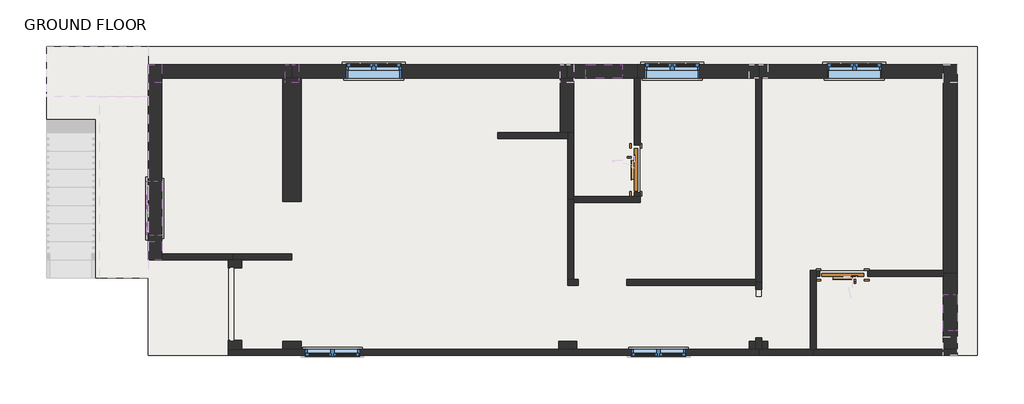
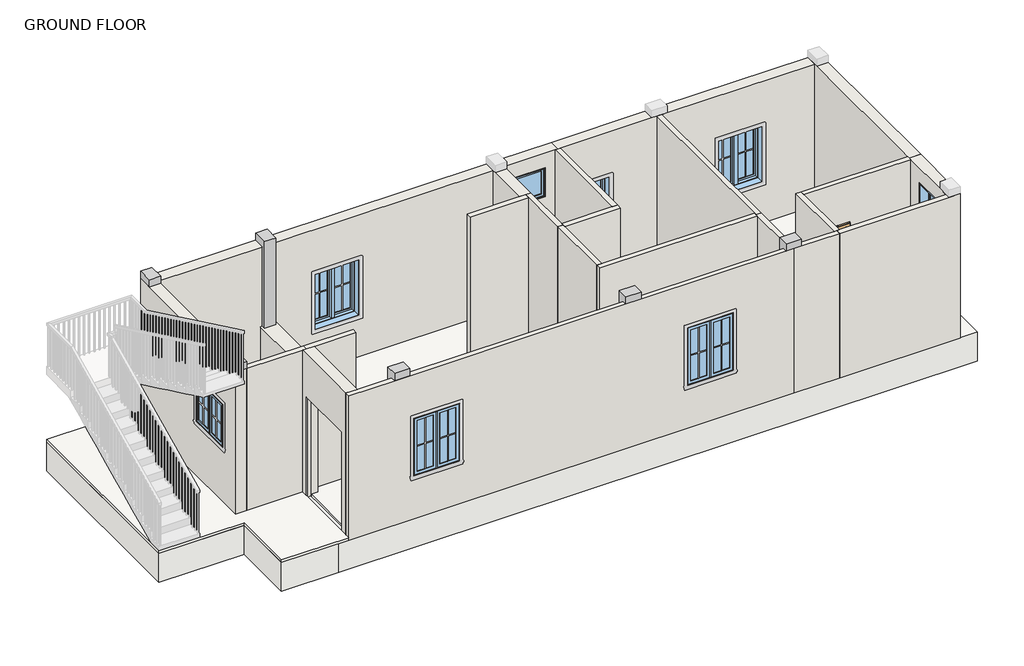
# One storey, part 1 of 3: 26 walls, 8 windows, 6 columns, 4 slabs, 2 doors.
"""IFC4 building model written with IfcOpenShell, lengths in millimetres."""

from ifc_helpers import new_model, si_unit, frame, origin, origin_with_axes, place, context, project, spatial, polyline, outline, extrude, faceted_brep, transform, mapped, element, save
from components import apartment_toilet_door_15897_d3_toilet_d7560075, apartment_toilet_door_15897_d3_toilet_03746f18, window_80340324, window_casement_double_w1_d341e8ac, window_casement_double_w1_80f1179f, window_casement_double_w1_2_90de19e9

model = new_model("IFC4")

# Units and contexts
model_context = context("Model", 3, world=origin())
ifc_project = project(units=[si_unit("LENGTHUNIT", "METRE", prefix="MILLI")], contexts=[model_context])

# Site, building, storey
site = spatial("IfcSite", under=ifc_project)
building = spatial("IfcBuilding", under=site)
storey = spatial("IfcBuildingStorey", under=building, Name="GROUND FLOOR", Elevation=0.0)

# Columns
placement = place(None, origin())
element("IfcColumn", 1, ObjectType="Rectangular Column : 9\" X 12\"", at=placement, inside=storey, context=model_context, shape_type="Brep", body=[
    faceted_brep([(-2166.0591227, 4797.7642852, 3200.4), (-2394.6591227, 4797.7642852, 3200.4), (-2394.6591227, 4797.7642852, 1371.6), (-2166.0591227, 4797.7642852, 1371.6), (-2394.6591227, 5102.5642852, 3200.4), (-2394.6591227, 5102.5642852, 3048.0), (-2394.6591227, 4873.9642852, 3048.0), (-2394.6591227, 4873.9642852, 1371.6), (-2166.0591227, 5102.5642852, 3200.4), (-2166.0591227, 5102.5642852, 3048.0), (-2280.3591227, 5102.5642852, 3048.0), (-2166.0591227, 4873.9642852, 1371.6), (-2166.0591227, 4873.9642852, 3048.0), (-2280.3591227, 4873.9642852, 3048.0), (-2280.3591227, 4873.9642852, 1371.6)], [[[0, 1, 2, 3]], [[1, 4, 5, 6, 7, 2]], [[4, 8, 9, 10, 5]], [[8, 0, 3, 11, 12, 9]], [[1, 0, 8, 4]], [[6, 13, 14, 7]], [[13, 6, 5, 10]], [[13, 12, 11, 14]], [[12, 13, 10, 9]], [[3, 2, 7, 14, 11]]]),
])
element("IfcColumn", 2, ObjectType="Rectangular Column : 9\" X 12\"", at=placement, inside=storey, context=model_context, shape_type="SweptSolid", body=[
    extrude(outline(polyline([(-4693.3591227, 5102.5642852), (-4464.7591227, 5102.5642852), (-4464.7591227, 4797.7642852), (-4693.3591227, 4797.7642852), (-4693.3591227, 5102.5642852)])), frame((0.0, 0.0, 3048.0), z_axis=(0.0, 0.0, 1.0), x_axis=(1.0, 0.0, 0.0)), (0.0, 0.0, 1.0), 152.4),
])
element("IfcColumn", 3, ObjectType="Rectangular Column : 9\" X 12\"", at=placement, inside=storey, context=model_context, shape_type="Brep", body=[
    faceted_brep([(5492.0408773, 454.3642852, 0.0), (5492.0408773, 327.3642852, 0.0), (5390.4408773, 327.3642852, 0.0), (5390.4408773, 454.3642852, 0.0), (5695.2408773, 454.3642852, 3200.4), (5695.2408773, 225.7642852, 3200.4), (5695.2408773, 225.7642852, 3048.0), (5695.2408773, 327.3642852, 3048.0), (5695.2408773, 327.3642852, 0.0), (5695.2408773, 454.3642852, 0.0), (5390.4408773, 225.7642852, 3200.4), (5390.4408773, 225.7642852, 3048.0), (5542.8408773, 225.7642852, 3048.0), (5390.4408773, 454.3642852, 3200.4), (5390.4408773, 327.3642852, 3048.0), (5593.6408773, 454.3642852, 0.0), (5593.6408773, 454.3642852, 3048.0), (5492.0408773, 454.3642852, 3048.0), (5593.6408773, 327.3642852, 3048.0), (5593.6408773, 327.3642852, 0.0), (5492.0408773, 327.3642852, 3048.0), (5542.8408773, 327.3642852, 3048.0)], [[[0, 1, 2, 3]], [[4, 5, 6, 7, 8, 9]], [[5, 10, 11, 12, 6]], [[10, 13, 3, 2, 14, 11]], [[4, 9, 15, 16, 17, 0, 3, 13]], [[5, 4, 13, 10]], [[18, 16, 15, 19]], [[17, 20, 1, 0]], [[16, 18, 21, 20, 17]], [[20, 14, 2, 1]], [[14, 20, 21, 12, 11]], [[7, 18, 19, 8]], [[18, 7, 6, 12, 21]], [[19, 15, 9, 8]]]),
])
element("IfcColumn", 4, ObjectType="Rectangular Column : 9\" X 12\"", at=placement, inside=storey, context=model_context, shape_type="SweptSolid", body=[
    extrude(outline(polyline([(225.7642852, 3200.4), (454.3642852, 3200.4), (454.3642852, 0.0), (327.3642852, 0.0), (327.3642852, 3048.0), (225.7642852, 3048.0), (225.7642852, 3200.4)])), frame((2190.0408773, 0.0, 0.0), z_axis=(1.0, 0.0, 0.0), x_axis=(0.0, 1.0, 0.0)), (0.0, 0.0, 1.0), 304.8),
])
element("IfcColumn", 5, ObjectType="Rectangular Column : 9\" X 12\"", at=placement, inside=storey, context=model_context, shape_type="SweptSolid", body=[
    extrude(outline(polyline([(225.7642852, 3200.4), (454.3642852, 3200.4), (454.3642852, 0.0), (327.3642852, 0.0), (327.3642852, 3048.0), (225.7642852, 3048.0), (225.7642852, 3200.4)])), frame((-2432.7591227, 0.0, 0.0), z_axis=(1.0, 0.0, 0.0), x_axis=(0.0, 1.0, 0.0)), (0.0, 0.0, 1.0), 304.8),
])
element("IfcColumn", 6, ObjectType="Rectangular Column : 9\" X 12\"", at=placement, inside=storey, context=model_context, shape_type="SweptSolid", body=[
    extrude(outline(polyline([(-4693.3591227, 2130.7642852), (-4464.7591227, 2130.7642852), (-4464.7591227, 1825.9642852), (-4693.3591227, 1825.9642852), (-4693.3591227, 2130.7642852)])), frame((0.0, 0.0, 3048.0), z_axis=(0.0, 0.0, 1.0), x_axis=(1.0, 0.0, 0.0)), (0.0, 0.0, 1.0), 152.4),
])

# Doors
apartment_toilet_door_15897_d3_toilet_shape = apartment_toilet_door_15897_d3_toilet_d7560075(model_context)
element("IfcDoor", 7, ObjectType="Apartment_Toilet_Door_15897 : D3 TOILET", at=placement, inside=storey, context=model_context, shape_type="MappedRepresentation", body=[
    mapped(apartment_toilet_door_15897_d3_toilet_shape, transform((6952.5408773, 1597.3642852, 0.0), x_axis=(-1.0, 0.0, 0.0), y_axis=(0.0, -1.0, 0.0), z_axis=(0.0, 0.0, 1.0))),
])
apartment_toilet_door_15897_d3_toilet_2_shape = apartment_toilet_door_15897_d3_toilet_03746f18(model_context)
element("IfcDoor", 8, ObjectType="Apartment_Toilet_Door_15897 : D3 TOILET", at=placement, inside=storey, context=model_context, shape_type="MappedRepresentation", body=[
    mapped(apartment_toilet_door_15897_d3_toilet_2_shape, transform((3510.8408773, 3337.2642852, 0.0), x_axis=(0.0, -1.0, 0.0), y_axis=(1.0, 0.0, 0.0), z_axis=(0.0, 0.0, 1.0))),
])

# Slabs
element("IfcSlab", 9, ObjectType="FLOORING", at=placement, inside=storey, context=model_context, shape_type="SweptSolid", body=[
    extrude(outline(polyline([(-4464.7591227, 1927.5642852), (-4464.7591227, 4873.9642852), (-2432.7591227, 4873.9642852), (-2432.7591227, 2803.8642852), (-2127.9591227, 2803.8642852), (-2127.9591227, 4873.9642852), (2215.4408773, 4873.9642852), (2215.4408773, 3959.5642852), (1174.0408773, 3959.5642852), (1174.0408773, 3857.9642852), (2342.4408773, 3857.9642852), (2342.4408773, 1394.1642852), (2520.2408773, 1394.1642852), (2520.2408773, 1495.7642852), (2444.0408773, 1495.7642852), (2444.0408773, 2791.1642852), (3561.6408773, 2791.1642852), (3561.6408773, 4873.9642852), (5492.0408773, 4873.9642852), (5492.0408773, 1495.7642852), (3409.2408773, 1495.7642852), (3333.0408773, 1495.7642852), (3333.0408773, 1394.1642852), (5492.0408773, 1394.1642852), (5492.0408773, 1203.6642852), (5593.6408773, 1203.6642852), (5593.6408773, 4873.9642852), (8641.6408773, 4873.9642852), (8641.6408773, 1648.1642852), (6406.4408773, 1648.1642852), (6406.4408773, 327.3642852), (5593.6408773, 327.3642852), (5593.6408773, 390.8642852), (5492.0408773, 390.8642852), (5492.0408773, 327.3642852), (-3118.5591227, 327.3642852), (-3118.5591227, 397.6642852), (-3250.1591227, 397.6642852), (-3250.1591227, 1769.2642852), (-3118.5591227, 1769.2642852), (-3118.5591227, 1825.9642852), (-2280.3591227, 1825.9642852), (-2280.3591227, 1927.5642852), (-4464.7591227, 1927.5642852)])), origin_with_axes(), (0.0, 0.0, 1.0), 50.8),
])
element("IfcSlab", 10, ObjectType="FLOORING OPEN AREA", at=placement, inside=storey, context=model_context, shape_type="SweptSolid", body=[
    extrude(outline(polyline([(-4693.3591227, 225.7642852), (-4693.3591227, 1521.1642852), (-6395.1591227, 1521.1642852), (-6395.1591227, 5407.3642852), (-4693.3591227, 5407.3642852), (-4693.3591227, 1825.9642852), (-3347.1591227, 1825.9642852), (-3347.1591227, 225.7642852), (-4693.3591227, 225.7642852)])), origin_with_axes(), (0.0, 0.0, 1.0), 50.8),
])
element("IfcSlab", 11, ObjectType="FLOORING TOILET", at=placement, inside=storey, context=model_context, shape_type="SweptSolid", body=[
    extrude(outline(polyline([(7371.5408773, 1546.5642852), (8641.6408773, 1546.5642852), (8641.6408773, 327.3642852), (6508.0408773, 327.3642852), (6508.0408773, 1546.5642852), (6571.5408773, 1546.5642852), (6571.5408773, 1648.1642852), (7371.5408773, 1648.1642852), (7371.5408773, 1546.5642852)])), origin_with_axes(), (0.0, 0.0, 1.0), 50.8),
    extrude(outline(polyline([(3460.0408773, 4873.9642852), (3460.0408773, 3756.2642852), (3561.6408773, 3756.2642852), (3561.6408773, 2956.2642852), (3460.0408773, 2956.2642852), (3460.0408773, 2892.7642852), (2444.0408773, 2892.7642852), (2444.0408773, 4873.9642852), (3460.0408773, 4873.9642852)])), origin_with_axes(), (0.0, 0.0, 1.0), 50.8),
])
element("IfcSlab", 12, ObjectType="Ground floor", at=placement, inside=storey, context=model_context, shape_type="SweptSolid", body=[
    extrude(outline(polyline([(9213.1408773, 5407.3642852), (9213.1408773, 225.7642852), (-3544.9797107, 225.7642852), (-4693.3591227, 225.7642852), (-4693.3591227, 1521.1642852), (-6395.1591227, 1521.1642852), (-6395.1591227, 5407.3642852), (9213.1408773, 5407.3642852)])), frame((0.0, 0.0, -609.6), z_axis=(0.0, 0.0, 1.0), x_axis=(1.0, 0.0, 0.0)), (0.0, 0.0, 1.0), 609.6),
])

# Walls
element("IfcWall", 13, at=placement, inside=storey, context=model_context, shape_type="Brep", body=[
    faceted_brep([(-2432.7591227, 4873.9642852, 0.0), (-2432.7591227, 2803.8642852, 0.0), (-2432.7591227, 2803.8642852, 1371.6), (-2432.7591227, 4873.9642852, 1371.6), (-2127.9591227, 4873.9642852, 0.0), (-2127.9591227, 4873.9642852, 1371.6), (-2127.9591227, 2803.8642852, 1371.6), (-2127.9591227, 2803.8642852, 0.0), (-2280.3591227, 4873.9642852, 0.0), (-2166.0591227, 4873.9642852, 1371.6), (-2280.3591227, 4873.9642852, 1371.6), (-2394.6591227, 4873.9642852, 1371.6)], [[[0, 1, 2, 3]], [[4, 5, 6, 7]], [[1, 0, 8, 4, 7]], [[2, 1, 7, 6]], [[3, 2, 6, 5, 9, 10, 11]], [[0, 3, 11, 10, 9, 5, 4, 8]]]),
])
element("IfcWall", 14, ObjectType="4\" WALL", at=placement, inside=storey, context=model_context, shape_type="Brep", body=[
    faceted_brep([(8870.2408773, 327.3642852, 0.0), (8641.6408773, 327.3642852, 0.0), (6508.0408773, 327.3642852, 0.0), (6457.2408773, 327.3642852, 0.0), (6457.2408773, 327.3642852, 3048.0), (6508.0408773, 327.3642852, 3048.0), (8641.6408773, 327.3642852, 3048.0), (8870.2408773, 327.3642852, 3048.0), (8870.2408773, 225.7642852, 0.0), (8870.2408773, 225.7642852, 3048.0), (8641.6408773, 225.7642852, 3048.0), (6457.2408773, 225.7642852, 3048.0), (6457.2408773, 225.7642852, 0.0)], [[[0, 1, 2, 3, 4, 5, 6, 7]], [[8, 9, 10, 11, 12]], [[3, 2, 1, 0, 8, 12]], [[4, 3, 12, 11]], [[0, 7, 9, 8]], [[7, 6, 5, 4, 11, 10, 9]]]),
])
element("IfcWall", 15, ObjectType="4\" WALL", at=placement, inside=storey, context=model_context, shape_type="Brep", body=[
    faceted_brep([(-2280.3591227, 1927.5642852, 0.0), (-3270.9591227, 1927.5642852, 0.0), (-3270.9591227, 1927.5642852, 3048.0), (-2280.3591227, 1927.5642852, 3048.0), (-2280.3591227, 1825.9642852, 0.0), (-2280.3591227, 1825.9642852, 3048.0), (-3118.5591227, 1825.9642852, 3048.0), (-3270.9591227, 1825.9642852, 3048.0), (-3270.9591227, 1825.9642852, 0.0), (-3118.5591227, 1825.9642852, 0.0)], [[[0, 1, 2, 3]], [[4, 5, 6, 7, 8, 9]], [[1, 0, 4, 9, 8]], [[2, 1, 8, 7]], [[0, 3, 5, 4]], [[3, 2, 7, 6, 5]]]),
])
element("IfcWall", 16, ObjectType="4\" WALL", at=placement, inside=storey, context=model_context, shape_type="Brep", body=[
    faceted_brep([(5593.6408773, 1444.9642852, 0.0), (5593.6408773, 1444.9642852, 3048.0), (5593.6408773, 454.3642852, 3048.0), (5593.6408773, 327.3642852, 3048.0), (5593.6408773, 327.3642852, 0.0), (5593.6408773, 454.3642852, 0.0), (5593.6408773, 517.8642852, 0.0), (5593.6408773, 517.8642852, 2133.6), (5593.6408773, 1330.6642852, 2133.6), (5593.6408773, 1330.6642852, 0.0), (5492.0408773, 1444.9642852, 3048.0), (5492.0408773, 1444.9642852, 0.0), (5492.0408773, 1394.1642852, 0.0), (5492.0408773, 1330.6642852, 0.0), (5492.0408773, 1330.6642852, 2133.6), (5492.0408773, 517.8642852, 2133.6), (5492.0408773, 517.8642852, 0.0), (5492.0408773, 454.3642852, 0.0), (5492.0408773, 327.3642852, 0.0), (5492.0408773, 327.3642852, 3048.0), (5492.0408773, 454.3642852, 3048.0), (5492.0408773, 1394.1642852, 3048.0), (5542.8408773, 327.3642852, 0.0), (5542.8408773, 327.3642852, 3048.0)], [[[0, 1, 2, 3, 4, 5, 6, 7, 8, 9]], [[10, 11, 12, 13, 14, 15, 16, 17, 18, 19, 20, 21]], [[11, 0, 9, 13, 12]], [[4, 22, 18, 17, 16, 6, 5]], [[1, 0, 11, 10]], [[4, 3, 23, 19, 18, 22]], [[15, 7, 6, 16]], [[7, 15, 14, 8]], [[8, 14, 13, 9]], [[3, 2, 1, 10, 21, 20, 19, 23]]]),
])
element("IfcWall", 17, ObjectType="4\" WALL", at=placement, inside=storey, context=model_context, shape_type="Brep", body=[
    faceted_brep([(5492.0408773, 1495.7642852, 0.0), (3333.0408773, 1495.7642852, 0.0), (3333.0408773, 1495.7642852, 2133.6), (2520.2408773, 1495.7642852, 2133.6), (2520.2408773, 1495.7642852, 0.0), (2444.0408773, 1495.7642852, 0.0), (2342.4408773, 1495.7642852, 0.0), (2342.4408773, 1495.7642852, 3048.0), (2444.0408773, 1495.7642852, 3048.0), (5492.0408773, 1495.7642852, 3048.0), (3333.0408773, 1394.1642852, 2133.6), (3333.0408773, 1394.1642852, 0.0), (5492.0408773, 1394.1642852, 0.0), (5492.0408773, 1394.1642852, 3048.0), (2342.4408773, 1394.1642852, 3048.0), (2342.4408773, 1394.1642852, 0.0), (2520.2408773, 1394.1642852, 0.0), (2520.2408773, 1394.1642852, 2133.6), (5492.0408773, 1444.9642852, 0.0), (5492.0408773, 1444.9642852, 3048.0)], [[[0, 1, 2, 3, 4, 5, 6, 7, 8, 9]], [[10, 11, 12, 13, 14, 15, 16, 17]], [[16, 15, 6, 5, 4]], [[12, 11, 1, 0, 18]], [[0, 9, 19, 13, 12, 18]], [[7, 6, 15, 14]], [[2, 1, 11, 10]], [[3, 2, 10, 17]], [[4, 3, 17, 16]], [[9, 8, 7, 14, 13, 19]]]),
])
element("IfcWall", 18, ObjectType="4\" WALL", at=placement, inside=storey, context=model_context, shape_type="Brep", body=[
    faceted_brep([(2444.0408773, 1495.7642852, 0.0), (2444.0408773, 2791.1642852, 0.0), (2444.0408773, 2841.9642852, 0.0), (2444.0408773, 2841.9642852, 3048.0), (2444.0408773, 2791.1642852, 3048.0), (2444.0408773, 1495.7642852, 3048.0), (2342.4408773, 1495.7642852, 0.0), (2342.4408773, 1495.7642852, 3048.0), (2342.4408773, 2841.9642852, 3048.0), (2342.4408773, 2841.9642852, 0.0)], [[[0, 1, 2, 3, 4, 5]], [[6, 7, 8, 9]], [[2, 1, 0, 6, 9]], [[3, 2, 9, 8]], [[0, 5, 7, 6]], [[5, 4, 3, 8, 7]]]),
])
element("IfcWall", 19, ObjectType="4\" WALL", at=placement, inside=storey, context=model_context, shape_type="Brep", body=[
    faceted_brep([(2342.4408773, 3959.5642852, 0.0), (2215.4408773, 3959.5642852, 0.0), (1174.0408773, 3959.5642852, 0.0), (1174.0408773, 3959.5642852, 3048.0), (2215.4408773, 3959.5642852, 3048.0), (2342.4408773, 3959.5642852, 3048.0), (2342.4408773, 3857.9642852, 0.0), (2342.4408773, 3857.9642852, 3048.0), (1174.0408773, 3857.9642852, 3048.0), (1174.0408773, 3857.9642852, 0.0)], [[[0, 1, 2, 3, 4, 5]], [[6, 7, 8, 9]], [[2, 1, 0, 6, 9]], [[3, 2, 9, 8]], [[0, 5, 7, 6]], [[5, 4, 3, 8, 7]]]),
])
element("IfcWall", 20, ObjectType="4\" WALL", at=placement, inside=storey, context=model_context, shape_type="Brep", body=[
    faceted_brep([(6508.0408773, 327.3642852, 0.0), (6508.0408773, 1546.5642852, 0.0), (6508.0408773, 1648.1642852, 0.0), (6508.0408773, 1648.1642852, 3048.0), (6508.0408773, 1546.5642852, 3048.0), (6508.0408773, 327.3642852, 3048.0), (6406.4408773, 327.3642852, 0.0), (6406.4408773, 327.3642852, 3048.0), (6406.4408773, 1648.1642852, 3048.0), (6406.4408773, 1648.1642852, 0.0), (6457.2408773, 327.3642852, 0.0), (6457.2408773, 327.3642852, 3048.0)], [[[0, 1, 2, 3, 4, 5]], [[6, 7, 8, 9]], [[2, 1, 0, 10, 6, 9]], [[0, 5, 11, 7, 6, 10]], [[3, 2, 9, 8]], [[5, 4, 3, 8, 7, 11]]]),
])
element("IfcWall", 21, ObjectType="4\" WALL", at=placement, inside=storey, context=model_context, shape_type="Brep", body=[
    faceted_brep([(6508.0408773, 1546.5642852, 0.0), (6571.5408773, 1546.5642852, 0.0), (6571.5408773, 1546.5642852, 2133.6), (7371.5408773, 1546.5642852, 2133.6), (7371.5408773, 1546.5642852, 0.0), (8641.6408773, 1546.5642852, 0.0), (8641.6408773, 1546.5642852, 3048.0), (6508.0408773, 1546.5642852, 3048.0), (6571.5408773, 1648.1642852, 2133.6), (6571.5408773, 1648.1642852, 0.0), (6508.0408773, 1648.1642852, 0.0), (6508.0408773, 1648.1642852, 3048.0), (8641.6408773, 1648.1642852, 3048.0), (8641.6408773, 1648.1642852, 0.0), (7371.5408773, 1648.1642852, 0.0), (7371.5408773, 1648.1642852, 2133.6), (8641.6408773, 1597.3642852, 0.0), (8641.6408773, 1597.3642852, 3048.0)], [[[0, 1, 2, 3, 4, 5, 6, 7]], [[8, 9, 10, 11, 12, 13, 14, 15]], [[14, 13, 16, 5, 4]], [[10, 9, 1, 0]], [[0, 7, 11, 10]], [[6, 5, 16, 13, 12, 17]], [[2, 1, 9, 8]], [[3, 2, 8, 15]], [[4, 3, 15, 14]], [[7, 6, 17, 12, 11]]]),
])
element("IfcWall", 22, ObjectType="4\" WALL", at=placement, inside=storey, context=model_context, shape_type="Brep", body=[
    faceted_brep([(2444.0408773, 2791.1642852, 0.0), (3561.6408773, 2791.1642852, 0.0), (3561.6408773, 2791.1642852, 3048.0), (2444.0408773, 2791.1642852, 3048.0), (2444.0408773, 2892.7642852, 0.0), (2444.0408773, 2892.7642852, 3048.0), (3460.0408773, 2892.7642852, 3048.0), (3561.6408773, 2892.7642852, 3048.0), (3561.6408773, 2892.7642852, 0.0), (3460.0408773, 2892.7642852, 0.0), (2444.0408773, 2841.9642852, 0.0), (2444.0408773, 2841.9642852, 3048.0)], [[[0, 1, 2, 3]], [[4, 5, 6, 7, 8, 9]], [[1, 0, 10, 4, 9, 8]], [[0, 3, 11, 5, 4, 10]], [[2, 1, 8, 7]], [[3, 2, 7, 6, 5, 11]]]),
])
element("IfcWall", 23, ObjectType="4\" WALL", at=placement, inside=storey, context=model_context, shape_type="Brep", body=[
    faceted_brep([(3561.6408773, 2892.7642852, 0.0), (3561.6408773, 2956.2642852, 0.0), (3561.6408773, 2956.2642852, 2133.6), (3561.6408773, 3756.2642852, 2133.6), (3561.6408773, 3756.2642852, 0.0), (3561.6408773, 4873.9642852, 0.0), (3561.6408773, 4873.9642852, 3048.0), (3561.6408773, 2892.7642852, 3048.0), (3460.0408773, 2956.2642852, 2133.6), (3460.0408773, 2956.2642852, 0.0), (3460.0408773, 2892.7642852, 0.0), (3460.0408773, 2892.7642852, 3048.0), (3460.0408773, 4873.9642852, 3048.0), (3460.0408773, 4873.9642852, 0.0), (3460.0408773, 3756.2642852, 0.0), (3460.0408773, 3756.2642852, 2133.6), (3510.8408773, 4873.9642852, 0.0), (3510.8408773, 4873.9642852, 3048.0)], [[[0, 1, 2, 3, 4, 5, 6, 7]], [[8, 9, 10, 11, 12, 13, 14, 15]], [[14, 13, 16, 5, 4]], [[10, 9, 1, 0]], [[0, 7, 11, 10]], [[6, 5, 16, 13, 12, 17]], [[2, 1, 9, 8]], [[3, 2, 8, 15]], [[4, 3, 15, 14]], [[7, 6, 17, 12, 11]]]),
])
element("IfcWall", 24, ObjectType="4\" WALL", at=placement, inside=storey, context=model_context, shape_type="Brep", body=[
    faceted_brep([(2444.0408773, 2841.9642852, 0.0), (2444.0408773, 2892.7642852, 0.0), (2444.0408773, 3959.5642852, 0.0), (2444.0408773, 3959.5642852, 3048.0), (2444.0408773, 2892.7642852, 3048.0), (2444.0408773, 2841.9642852, 3048.0), (2342.4408773, 2841.9642852, 0.0), (2342.4408773, 2841.9642852, 3048.0), (2342.4408773, 3857.9642852, 3048.0), (2342.4408773, 3959.5642852, 3048.0), (2342.4408773, 3959.5642852, 0.0), (2342.4408773, 3857.9642852, 0.0)], [[[0, 1, 2, 3, 4, 5]], [[6, 7, 8, 9, 10, 11]], [[2, 1, 0, 6, 11, 10]], [[0, 5, 7, 6]], [[5, 4, 3, 9, 8, 7]], [[3, 2, 10, 9]]]),
])
element("IfcWall", 25, ObjectType="4\" WALL", at=placement, inside=storey, context=model_context, shape_type="SweptSolid", body=[
    extrude(outline(polyline([(-4464.7591227, 1927.5642852), (-3270.9591227, 1927.5642852), (-3270.9591227, 1825.9642852), (-4464.7591227, 1825.9642852), (-4464.7591227, 1927.5642852)])), origin_with_axes(), (0.0, 0.0, 1.0), 3048.0),
])
element("IfcWall", 26, ObjectType="4\" WALL", at=placement, inside=storey, context=model_context, shape_type="Brep", body=[
    faceted_brep([(5593.6408773, 1444.9642852, 0.0), (5593.6408773, 4873.9642852, 0.0), (5593.6408773, 4873.9642852, 3048.0), (5593.6408773, 1444.9642852, 3048.0), (5492.0408773, 1444.9642852, 0.0), (5492.0408773, 1444.9642852, 3048.0), (5492.0408773, 1495.7642852, 3048.0), (5492.0408773, 4873.9642852, 3048.0), (5492.0408773, 4873.9642852, 0.0), (5492.0408773, 1495.7642852, 0.0), (5542.8408773, 4873.9642852, 0.0), (5542.8408773, 4873.9642852, 3048.0)], [[[0, 1, 2, 3]], [[4, 5, 6, 7, 8, 9]], [[1, 0, 4, 9, 8, 10]], [[0, 3, 5, 4]], [[2, 1, 10, 8, 7, 11]], [[3, 2, 11, 7, 6, 5]]]),
])
element("IfcWall", 27, ObjectType="4\" WALL", at=placement, inside=storey, context=model_context, shape_type="Brep", body=[
    faceted_brep([(5542.8408773, 327.3642852, 0.0), (5492.0408773, 327.3642852, 0.0), (5390.4408773, 327.3642852, 0.0), (2494.8408773, 327.3642852, 0.0), (2190.0408773, 327.3642852, 0.0), (-2127.9591227, 327.3642852, 0.0), (-2432.7591227, 327.3642852, 0.0), (-3118.5591227, 327.3642852, 0.0), (-3347.1591227, 327.3642852, 0.0), (-3347.1591227, 327.3642852, 3048.0), (-3118.5591227, 327.3642852, 3048.0), (-2432.7591227, 327.3642852, 3048.0), (-2127.9591227, 327.3642852, 3048.0), (2190.0408773, 327.3642852, 3048.0), (2494.8408773, 327.3642852, 3048.0), (5390.4408773, 327.3642852, 3048.0), (5492.0408773, 327.3642852, 3048.0), (5542.8408773, 327.3642852, 3048.0), (3409.2408773, 327.3642852, 2133.6), (3409.2408773, 327.3642852, 914.4), (4323.6408773, 327.3642852, 914.4), (4323.6408773, 327.3642852, 2133.6), (-2058.1091227, 327.3642852, 2133.6), (-2058.1091227, 327.3642852, 914.4), (-1143.7091227, 327.3642852, 914.4), (-1143.7091227, 327.3642852, 2133.6), (5542.8408773, 225.7642852, 0.0), (5542.8408773, 225.7642852, 3048.0), (5390.4408773, 225.7642852, 3048.0), (2494.8408773, 225.7642852, 3048.0), (2190.0408773, 225.7642852, 3048.0), (-2127.9591227, 225.7642852, 3048.0), (-2432.7591227, 225.7642852, 3048.0), (-3347.1591227, 225.7642852, 3048.0), (-3347.1591227, 225.7642852, 0.0), (3409.2408773, 225.7642852, 2133.6), (4323.6408773, 225.7642852, 2133.6), (4323.6408773, 225.7642852, 914.4), (3409.2408773, 225.7642852, 914.4), (-2058.1091227, 225.7642852, 2133.6), (-1143.7091227, 225.7642852, 2133.6), (-1143.7091227, 225.7642852, 914.4), (-2058.1091227, 225.7642852, 914.4)], [[[0, 1, 2, 3, 4, 5, 6, 7, 8, 9, 10, 11, 12, 13, 14, 15, 16, 17], [18, 19, 20, 21], [22, 23, 24, 25]], [[26, 27, 28, 29, 30, 31, 32, 33, 34], [35, 36, 37, 38], [39, 40, 41, 42]], [[8, 7, 6, 5, 4, 3, 2, 1, 0, 26, 34]], [[0, 17, 27, 26]], [[9, 8, 34, 33]], [[18, 21, 36, 35]], [[21, 20, 37, 36]], [[20, 19, 38, 37]], [[19, 18, 35, 38]], [[22, 25, 40, 39]], [[25, 24, 41, 40]], [[24, 23, 42, 41]], [[23, 22, 39, 42]], [[17, 16, 15, 14, 13, 12, 11, 10, 9, 33, 32, 31, 30, 29, 28, 27]]]),
])
element("IfcWall", 28, ObjectType="4\" WALL", at=placement, inside=storey, context=model_context, shape_type="Brep", body=[
    faceted_brep([(6457.2408773, 327.3642852, 0.0), (6406.4408773, 327.3642852, 0.0), (5695.2408773, 327.3642852, 0.0), (5593.6408773, 327.3642852, 0.0), (5542.8408773, 327.3642852, 0.0), (5542.8408773, 327.3642852, 3048.0), (5593.6408773, 327.3642852, 3048.0), (5695.2408773, 327.3642852, 3048.0), (6406.4408773, 327.3642852, 3048.0), (6457.2408773, 327.3642852, 3048.0), (6457.2408773, 225.7642852, 0.0), (6457.2408773, 225.7642852, 3048.0), (5695.2408773, 225.7642852, 3048.0), (5542.8408773, 225.7642852, 3048.0), (5542.8408773, 225.7642852, 0.0)], [[[0, 1, 2, 3, 4, 5, 6, 7, 8, 9]], [[10, 11, 12, 13, 14]], [[4, 3, 2, 1, 0, 10, 14]], [[5, 4, 14, 13]], [[0, 9, 11, 10]], [[9, 8, 7, 6, 5, 13, 12, 11]]]),
])
element("IfcWall", 29, ObjectType="9\"", at=placement, inside=storey, context=model_context, shape_type="Brep", body=[
    faceted_brep([(2444.0408773, 3959.5642852, 0.0), (2444.0408773, 4873.9642852, 0.0), (2444.0408773, 4873.9642852, 3048.0), (2444.0408773, 4797.7642852, 3048.0), (2444.0408773, 3959.5642852, 3048.0), (2215.4408773, 3959.5642852, 0.0), (2215.4408773, 3959.5642852, 3048.0), (2215.4408773, 4797.7642852, 3048.0), (2215.4408773, 4873.9642852, 3048.0), (2215.4408773, 4873.9642852, 0.0), (2342.4408773, 3959.5642852, 0.0), (2329.7408773, 4873.9642852, 0.0), (2342.4408773, 3959.5642852, 3048.0), (2329.7408773, 4873.9642852, 3048.0)], [[[0, 1, 2, 3, 4]], [[5, 6, 7, 8, 9]], [[1, 0, 10, 5, 9, 11]], [[0, 4, 12, 6, 5, 10]], [[4, 3, 2, 13, 8, 7, 6, 12]], [[2, 1, 11, 9, 8, 13]]]),
])
element("IfcWall", 30, ObjectType="9\" WALL", at=placement, inside=storey, context=model_context, shape_type="Brep", body=[
    faceted_brep([(8641.6408773, 5102.5642852, 0.0), (5542.8408773, 5102.5642852, 0.0), (5542.8408773, 5102.5642852, 3048.0), (5695.2408773, 5102.5642852, 3048.0), (8641.6408773, 5102.5642852, 3048.0), (7606.5908773, 5102.5642852, 2133.6), (6692.1908773, 5102.5642852, 2133.6), (6692.1908773, 5102.5642852, 914.4), (7606.5908773, 5102.5642852, 914.4), (8641.6408773, 4873.9642852, 0.0), (8641.6408773, 4873.9642852, 3048.0), (5695.2408773, 4873.9642852, 3048.0), (5593.6408773, 4873.9642852, 3048.0), (5542.8408773, 4873.9642852, 3048.0), (5542.8408773, 4873.9642852, 0.0), (5593.6408773, 4873.9642852, 0.0), (7606.5908773, 4873.9642852, 2133.6), (7606.5908773, 4873.9642852, 914.4), (6692.1908773, 4873.9642852, 914.4), (6692.1908773, 4873.9642852, 2133.6)], [[[0, 1, 2, 3, 4], [5, 6, 7, 8]], [[9, 10, 11, 12, 13, 14, 15], [16, 17, 18, 19]], [[1, 0, 9, 15, 14]], [[2, 1, 14, 13]], [[0, 4, 10, 9]], [[17, 16, 5, 8]], [[18, 17, 8, 7]], [[19, 18, 7, 6]], [[16, 19, 6, 5]], [[4, 3, 2, 13, 12, 11, 10]]]),
])
element("IfcWall", 31, ObjectType="9\" WALL", at=placement, inside=storey, context=model_context, shape_type="Brep", body=[
    faceted_brep([(8870.2408773, 327.3642852, 0.0), (8870.2408773, 1597.3642852, 0.0), (8870.2408773, 1597.3642852, 3048.0), (8870.2408773, 530.5642852, 3048.0), (8870.2408773, 327.3642852, 3048.0), (8870.2408773, 632.1642852, 2743.2), (8870.2408773, 1241.7642852, 2743.2), (8870.2408773, 1241.7642852, 2133.6), (8870.2408773, 632.1642852, 2133.6), (8641.6408773, 327.3642852, 0.0), (8641.6408773, 327.3642852, 3048.0), (8641.6408773, 530.5642852, 3048.0), (8641.6408773, 1546.5642852, 3048.0), (8641.6408773, 1597.3642852, 3048.0), (8641.6408773, 1597.3642852, 0.0), (8641.6408773, 1546.5642852, 0.0), (8641.6408773, 632.1642852, 2743.2), (8641.6408773, 632.1642852, 2133.6), (8641.6408773, 1241.7642852, 2133.6), (8641.6408773, 1241.7642852, 2743.2)], [[[0, 1, 2, 3, 4], [5, 6, 7, 8]], [[9, 10, 11, 12, 13, 14, 15], [16, 17, 18, 19]], [[1, 0, 9, 15, 14]], [[2, 1, 14, 13]], [[0, 4, 10, 9]], [[17, 16, 5, 8]], [[18, 17, 8, 7]], [[19, 18, 7, 6]], [[16, 19, 6, 5]], [[4, 3, 2, 13, 12, 11, 10]]]),
])
element("IfcWall", 32, ObjectType="9\" WALL", at=placement, inside=storey, context=model_context, shape_type="Brep", body=[
    faceted_brep([(-4464.7591227, 1825.9642852, 0.0), (-4464.7591227, 1927.5642852, 0.0), (-4464.7591227, 4873.9642852, 0.0), (-4464.7591227, 5102.5642852, 0.0), (-4464.7591227, 5102.5642852, 3048.0), (-4464.7591227, 4873.9642852, 3048.0), (-4464.7591227, 4797.7642852, 3048.0), (-4464.7591227, 2130.7642852, 3048.0), (-4464.7591227, 1927.5642852, 3048.0), (-4464.7591227, 1825.9642852, 3048.0), (-4464.7591227, 3146.7642852, 2133.6), (-4464.7591227, 3146.7642852, 1219.2), (-4464.7591227, 2232.3642852, 1219.2), (-4464.7591227, 2232.3642852, 2133.6), (-4693.3591227, 1825.9642852, 0.0), (-4693.3591227, 1825.9642852, 3048.0), (-4693.3591227, 2130.7642852, 3048.0), (-4693.3591227, 4797.7642852, 3048.0), (-4693.3591227, 5102.5642852, 3048.0), (-4693.3591227, 5102.5642852, 0.0), (-4693.3591227, 3146.7642852, 2133.6), (-4693.3591227, 2232.3642852, 2133.6), (-4693.3591227, 2232.3642852, 1219.2), (-4693.3591227, 3146.7642852, 1219.2)], [[[0, 1, 2, 3, 4, 5, 6, 7, 8, 9], [10, 11, 12, 13]], [[14, 15, 16, 17, 18, 19], [20, 21, 22, 23]], [[3, 2, 1, 0, 14, 19]], [[4, 3, 19, 18]], [[0, 9, 15, 14]], [[11, 10, 20, 23]], [[12, 11, 23, 22]], [[13, 12, 22, 21]], [[10, 13, 21, 20]], [[9, 8, 7, 6, 5, 4, 18, 17, 16, 15]]]),
])
element("IfcWall", 33, ObjectType="9\" WALL", at=placement, inside=storey, context=model_context, shape_type="Brep", body=[
    faceted_brep([(-3118.5591227, 327.3642852, 3048.0), (-3118.5591227, 327.3642852, 0.0), (-3118.5591227, 473.8642852, 0.0), (-3118.5591227, 473.8642852, 2133.6), (-3118.5591227, 1693.0642852, 2133.6), (-3118.5591227, 1693.0642852, 0.0), (-3118.5591227, 1825.9642852, 0.0), (-3118.5591227, 1825.9642852, 3048.0), (-3347.1591227, 327.3642852, 0.0), (-3347.1591227, 327.3642852, 3048.0), (-3347.1591227, 1825.9642852, 3048.0), (-3347.1591227, 1825.9642852, 0.0), (-3347.1591227, 1693.0642852, 0.0), (-3347.1591227, 1693.0642852, 2133.6), (-3347.1591227, 473.8642852, 2133.6), (-3347.1591227, 473.8642852, 0.0), (-3327.1591227, 473.8642852, 0.0), (-3327.1591227, 458.8642852, 0.0), (-3250.1591227, 458.8642852, 0.0), (-3250.1591227, 473.8642852, 0.0), (-3270.9591227, 1825.9642852, 0.0), (-3250.1591227, 1693.0642852, 0.0), (-3250.1591227, 1708.0642852, 0.0), (-3327.1591227, 1708.0642852, 0.0), (-3327.1591227, 1693.0642852, 0.0), (-3270.9591227, 1825.9642852, 3048.0), (-3327.1591227, 1693.0642852, 2133.6), (-3327.1591227, 473.8642852, 2133.6), (-3327.1591227, 1708.0642852, 2148.6), (-3327.1591227, 458.8642852, 2148.6), (-3250.1591227, 1708.0642852, 2148.6), (-3250.1591227, 1693.0642852, 2133.6), (-3250.1591227, 473.8642852, 2133.6), (-3250.1591227, 458.8642852, 2148.6)], [[[0, 1, 2, 3, 4, 5, 6, 7]], [[8, 9, 10, 11, 12, 13, 14, 15]], [[1, 8, 15, 16, 17, 18, 19, 2]], [[11, 20, 6, 5, 21, 22, 23, 24, 12]], [[1, 0, 9, 8]], [[7, 6, 20, 11, 10, 25]], [[24, 26, 13, 12]], [[27, 16, 15, 14]], [[26, 27, 14, 13]], [[26, 24, 23, 28, 29, 17, 16, 27]], [[28, 23, 22, 30]], [[30, 22, 21, 31, 32, 19, 18, 33]], [[29, 28, 30, 33]], [[17, 29, 33, 18]], [[31, 21, 5, 4]], [[19, 32, 3, 2]], [[32, 31, 4, 3]], [[0, 7, 25, 10, 9]]]),
])
element("IfcWall", 34, ObjectType="9\" WALL", at=placement, inside=storey, context=model_context, shape_type="Brep", body=[
    faceted_brep([(-2280.3591227, 5102.5642852, 3048.0), (-2280.3591227, 5102.5642852, 0.0), (-4464.7591227, 5102.5642852, 0.0), (-4464.7591227, 5102.5642852, 3048.0), (-2394.6591227, 5102.5642852, 3048.0), (-2280.3591227, 4873.9642852, 0.0), (-2280.3591227, 4873.9642852, 3048.0), (-2394.6591227, 4873.9642852, 3048.0), (-4464.7591227, 4873.9642852, 3048.0), (-4464.7591227, 4873.9642852, 0.0), (-2432.7591227, 4873.9642852, 0.0)], [[[0, 1, 2, 3, 4]], [[5, 6, 7, 8, 9, 10]], [[2, 1, 5, 10, 9]], [[3, 2, 9, 8]], [[0, 6, 5, 1]], [[0, 4, 3, 8, 7, 6]]]),
])
element("IfcWall", 35, ObjectType="9\" WALL", at=placement, inside=storey, context=model_context, shape_type="Brep", body=[
    faceted_brep([(2329.7408773, 5102.5642852, 0.0), (-2280.3591227, 5102.5642852, 0.0), (-2280.3591227, 5102.5642852, 3048.0), (-2166.0591227, 5102.5642852, 3048.0), (2215.4408773, 5102.5642852, 3048.0), (2329.7408773, 5102.5642852, 3048.0), (-451.5591227, 5102.5642852, 2133.6), (-1365.9591227, 5102.5642852, 2133.6), (-1365.9591227, 5102.5642852, 914.4), (-451.5591227, 5102.5642852, 914.4), (2329.7408773, 4873.9642852, 0.0), (2329.7408773, 4873.9642852, 3048.0), (2215.4408773, 4873.9642852, 3048.0), (-2166.0591227, 4873.9642852, 3048.0), (-2280.3591227, 4873.9642852, 3048.0), (-2280.3591227, 4873.9642852, 0.0), (-2127.9591227, 4873.9642852, 0.0), (2215.4408773, 4873.9642852, 0.0), (-451.5591227, 4873.9642852, 2133.6), (-451.5591227, 4873.9642852, 914.4), (-1365.9591227, 4873.9642852, 914.4), (-1365.9591227, 4873.9642852, 2133.6)], [[[0, 1, 2, 3, 4, 5], [6, 7, 8, 9]], [[10, 11, 12, 13, 14, 15, 16, 17], [18, 19, 20, 21]], [[1, 0, 10, 17, 16, 15]], [[0, 5, 11, 10]], [[1, 15, 14, 2]], [[18, 21, 7, 6]], [[21, 20, 8, 7]], [[20, 19, 9, 8]], [[19, 18, 6, 9]], [[5, 4, 3, 2, 14, 13, 12, 11]]]),
])
element("IfcWall", 36, ObjectType="9\" WALL", at=placement, inside=storey, context=model_context, shape_type="Brep", body=[
    faceted_brep([(5542.8408773, 5102.5642852, 0.0), (3510.8408773, 5102.5642852, 0.0), (3510.8408773, 5102.5642852, 3048.0), (5390.4408773, 5102.5642852, 3048.0), (5542.8408773, 5102.5642852, 3048.0), (4552.2408773, 5102.5642852, 2133.6), (3637.8408773, 5102.5642852, 2133.6), (3637.8408773, 5102.5642852, 914.4), (4552.2408773, 5102.5642852, 914.4), (5542.8408773, 4873.9642852, 0.0), (5542.8408773, 4873.9642852, 3048.0), (5492.0408773, 4873.9642852, 3048.0), (5390.4408773, 4873.9642852, 3048.0), (3561.6408773, 4873.9642852, 3048.0), (3510.8408773, 4873.9642852, 3048.0), (3510.8408773, 4873.9642852, 0.0), (3561.6408773, 4873.9642852, 0.0), (5492.0408773, 4873.9642852, 0.0), (4552.2408773, 4873.9642852, 2133.6), (4552.2408773, 4873.9642852, 914.4), (3637.8408773, 4873.9642852, 914.4), (3637.8408773, 4873.9642852, 2133.6)], [[[0, 1, 2, 3, 4], [5, 6, 7, 8]], [[9, 10, 11, 12, 13, 14, 15, 16, 17], [18, 19, 20, 21]], [[1, 0, 9, 17, 16, 15]], [[2, 1, 15, 14]], [[0, 4, 10, 9]], [[18, 21, 6, 5]], [[21, 20, 7, 6]], [[20, 19, 8, 7]], [[19, 18, 5, 8]], [[4, 3, 2, 14, 13, 12, 11, 10]]]),
])
element("IfcWall", 37, ObjectType="9\" WALL", at=placement, inside=storey, context=model_context, shape_type="Brep", body=[
    faceted_brep([(8870.2408773, 1597.3642852, 0.0), (8870.2408773, 5102.5642852, 0.0), (8870.2408773, 5102.5642852, 3048.0), (8870.2408773, 4797.7642852, 3048.0), (8870.2408773, 1597.3642852, 3048.0), (8641.6408773, 1597.3642852, 0.0), (8641.6408773, 1597.3642852, 3048.0), (8641.6408773, 1648.1642852, 3048.0), (8641.6408773, 4797.7642852, 3048.0), (8641.6408773, 4873.9642852, 3048.0), (8641.6408773, 5102.5642852, 3048.0), (8641.6408773, 5102.5642852, 0.0), (8641.6408773, 4873.9642852, 0.0), (8641.6408773, 1648.1642852, 0.0)], [[[0, 1, 2, 3, 4]], [[5, 6, 7, 8, 9, 10, 11, 12, 13]], [[1, 0, 5, 13, 12, 11]], [[0, 4, 6, 5]], [[2, 1, 11, 10]], [[4, 3, 2, 10, 9, 8, 7, 6]]]),
])
element("IfcWall", 38, ObjectType="9\" WALL", at=placement, inside=storey, context=model_context, shape_type="Brep", body=[
    faceted_brep([(3510.8408773, 5102.5642852, 0.0), (2329.7408773, 5102.5642852, 0.0), (2329.7408773, 5102.5642852, 3048.0), (2444.0408773, 5102.5642852, 3048.0), (3510.8408773, 5102.5642852, 3048.0), (2647.2408773, 5102.5642852, 2743.2), (2647.2408773, 5102.5642852, 2133.6), (3256.8408773, 5102.5642852, 2133.6), (3256.8408773, 5102.5642852, 2743.2), (3510.8408773, 4873.9642852, 0.0), (3510.8408773, 4873.9642852, 3048.0), (3460.0408773, 4873.9642852, 3048.0), (2444.0408773, 4873.9642852, 3048.0), (2329.7408773, 4873.9642852, 3048.0), (2329.7408773, 4873.9642852, 0.0), (2444.0408773, 4873.9642852, 0.0), (3460.0408773, 4873.9642852, 0.0), (2647.2408773, 4873.9642852, 2743.2), (3256.8408773, 4873.9642852, 2743.2), (3256.8408773, 4873.9642852, 2133.6), (2647.2408773, 4873.9642852, 2133.6)], [[[0, 1, 2, 3, 4], [5, 6, 7, 8]], [[9, 10, 11, 12, 13, 14, 15, 16], [17, 18, 19, 20]], [[1, 0, 9, 16, 15, 14]], [[2, 1, 14, 13]], [[0, 4, 10, 9]], [[5, 8, 18, 17]], [[8, 7, 19, 18]], [[7, 6, 20, 19]], [[6, 5, 17, 20]], [[4, 3, 2, 13, 12, 11, 10]]]),
])

# Windows
window_shape = window_80340324(model_context)
element("IfcWindow", 39, ObjectType="Fixed : 24\" x 24\"", at=placement, inside=storey, context=model_context, shape_type="MappedRepresentation", body=[
    mapped(window_shape, transform((2913.9408773, 4988.2642852, 1219.2), x_axis=(-1.0, 0.0, 0.0), y_axis=(0.0, -1.0, 0.0), z_axis=(0.0, 0.0, 1.0))),
])
element("IfcWindow", 40, ObjectType="Fixed : 24\" x 24\"", at=placement, inside=storey, context=model_context, shape_type="MappedRepresentation", body=[
    mapped(window_shape, transform((8755.9408773, 898.8642852, 1219.2), x_axis=(0.0, -1.0, 0.0), y_axis=(1.0, 0.0, 0.0), z_axis=(0.0, 0.0, 1.0))),
])
window_casement_double_w1_shape = window_casement_double_w1_d341e8ac(model_context)
element("IfcWindow", 41, ObjectType="Window-Casement-Double : w1", at=placement, inside=storey, context=model_context, shape_type="MappedRepresentation", body=[
    mapped(window_casement_double_w1_shape, transform((-908.7591227, 4988.2642852, 0.0), x_axis=(1.0, 0.0, 0.0), y_axis=(0.0, 1.0, 0.0), z_axis=(0.0, 0.0, 1.0))),
])
element("IfcWindow", 42, ObjectType="Window-Casement-Double : w1", at=placement, inside=storey, context=model_context, shape_type="MappedRepresentation", body=[
    mapped(window_casement_double_w1_shape, transform((4095.0408773, 4988.2642852, 0.0), x_axis=(1.0, 0.0, 0.0), y_axis=(0.0, 1.0, 0.0), z_axis=(0.0, 0.0, 1.0))),
])
element("IfcWindow", 43, ObjectType="Window-Casement-Double : w1", at=placement, inside=storey, context=model_context, shape_type="MappedRepresentation", body=[
    mapped(window_casement_double_w1_shape, transform((7149.3908773, 4988.2642852, 0.0), x_axis=(1.0, 0.0, 0.0), y_axis=(0.0, 1.0, 0.0), z_axis=(0.0, 0.0, 1.0))),
])
window_casement_double_w1_2_shape = window_casement_double_w1_80f1179f(model_context)
element("IfcWindow", 44, ObjectType="Window-Casement-Double : w1", at=placement, inside=storey, context=model_context, shape_type="MappedRepresentation", body=[
    mapped(window_casement_double_w1_2_shape, transform((3866.4408773, 276.5642852, 0.0), x_axis=(-1.0, 0.0, 0.0), y_axis=(0.0, -1.0, 0.0), z_axis=(0.0, 0.0, 1.0))),
])
element("IfcWindow", 45, ObjectType="Window-Casement-Double : w1", at=placement, inside=storey, context=model_context, shape_type="MappedRepresentation", body=[
    mapped(window_casement_double_w1_2_shape, transform((-1600.9091227, 276.5642852, 0.0), x_axis=(-1.0, 0.0, 0.0), y_axis=(0.0, -1.0, 0.0), z_axis=(0.0, 0.0, 1.0))),
])
window_casement_double_w1_2_2_shape = window_casement_double_w1_2_90de19e9(model_context)
element("IfcWindow", 46, ObjectType="Window-Casement-Double : w1 2", at=placement, inside=storey, context=model_context, shape_type="MappedRepresentation", body=[
    mapped(window_casement_double_w1_2_2_shape, transform((-4579.0591227, 2689.5642852, 304.8), x_axis=(0.0, 1.0, 0.0), y_axis=(-1.0, 0.0, 0.0), z_axis=(0.0, 0.0, 1.0))),
])

save(model, "model.ifc")

# Revit data of these elements
# Type "Rectangular Column : 9\" X 12\""
#   Assembly Code = "B1010200"
#   Depth = 0' - 9"
#   Offset Base = 0' - 0"
#   Offset Top = 0' - 0"
#   Width = 1' - 0"
#   Material = none
# Type "Apartment_Toilet_Door_15897 : D3 TOILET"
#   Type Mark = "15"
#   Panel Type = ""
#   Location [instance default] = ""
#   Door Type = "Semi Solid Flushed Wooden Door Laminated on Boths Sides- Bathroom / Laundry"
#   Construction Type Id = "DOOR"
#   Analytic Construction = "Wooden"
#   Threshold Depth = 0' - 1.1811"
#   Thickness = 0' - 2.12598"
#   Thermal Resistance (R) = 2.58758 (h·ft²·°F)/BTU
#   Heat Transfer Coefficient (U) = 0.386456 BTU/(h·ft²·°F)
#   Height = 7' - 0"
#   Trim Projection Ext = 0' - 0.98425"
#   Trim Projection Int = 0' - 0.98425"
#   Width = 2' - 6"
#   Define Thermal Properties by = 1
#   Threshold Material = BEL-Threshold material-Marble
#   Visual Light Transmittance = 0
#   Solar Heat Gain Coefficient = 0
#   Function = (empty or 0)
#   Wall Closure = (empty or 0)
# Type "FLOORING"
#   Assembly Code = "B1010"
#   Function = 0
#   Layers, outside or top first: 0' - 2" "FLOORING" (function 1)
# Type "FLOORING OPEN AREA"
#   Assembly Code = "B1010"
#   Function = 0
#   Layers, outside or top first: 0' - 2" "OPEN AREA TILE" (function 1)
# Type "FLOORING TOILET"
#   Assembly Code = "B1010"
#   Function = 0
#   Layers, outside or top first: 0' - 2" "toilet wash room" (function 1)
# Type "Ground floor"
#   Assembly Code = "B1010"
#   Function = 0
#   Layers, outside or top first: 2' - 0" no material (function 1)
# Type
#   Assembly Code = "B2010"
#   Layers, outside or top first: 1' - 0" "Brick, Common" (function 1)
# Type "4\" WALL"
#   Assembly Code = "B2010"
#   Layers, outside or top first: 0' - 4" "Brick, Common" (function 1)
# Type "9\""
#   Assembly Code = "B2010"
#   Layers, outside or top first: 0' - 9" "Brick, Common" (function 1)
# Type "9\" WALL"
#   Assembly Code = "B2010"
#   Layers, outside or top first: 0' - 9" "Brick, Common" (function 1)
# Type "Fixed : 24\" x 24\""
#   Type Mark = "4"
#   Construction Type Id = "GSP4R"
#   Assembly Code = "B2020100"
#   Analytic Construction = "1/8 in Pilkington single glazing"
#   Visual Light Transmittance = 0.9
#   Solar Heat Gain Coefficient = 0.78
#   Heat Transfer Coefficient (U) = 0.6496 BTU/(h·ft²·°F)
#   Height = 2' - 0"
#   Default Sill Height = 3' - 0"
#   Width = 2' - 0"
#   Window Inset = 0' - 0 3/4"
#   Define Thermal Properties by = 1
#   Define Thermal Properties by = 1
#   Glass Pane Material = Glass
#   Sash Material = Sash
#   Wall Closure = (empty or 0)
# Type "Window-Casement-Double : w1"
#   Type Mark = "14"
#   Fire Rating = "0.5h"
#   Assembly Code = "B2020100"
#   Analytic Construction = "Double glazing - domestic"
#   Frame Extension [instance default] = 0' - 0 1/4"
#   Window Inset [instance default] = 0' - 0"
#   Wall Thickness [instance default] = 0' - 6"
#   Interior Wall Closure [instance default] = 0' - 2 1/4"
#   Half Width = 1' - 6"
#   Visual Light Transmittance = 0.81
#   Thermal Resistance (R) = 1.8146 (h·ft²·°F)/BTU
#   Solar Heat Gain Coefficient = 0.76
#   Rough Width = 3' - 0 1/2"
#   Rough Height = 4' - 0 1/2"
#   Height = 4' - 0"
#   Heat Transfer Coefficient (U) = 0.5511 BTU/(h·ft²·°F)
#   Exterior Wall Closure [instance default] = 0' - 1 1/4"
#   Extension Jamb [instance default] = 0' - 2 1/4"
#   Default Sill Height = 3' - 0"
#   Width = 3' - 0"
#   Define Thermal Properties by = 0
#   Muntin Visibility = yes
#   Interior Trim Visibility [instance default] = yes
#   Exterior Trim Visibility [instance default] = yes
#   Extension Jamb Visibility [instance default] = yes
#   Muntin Pattern = Muntin Pattern_2x2 : Muntin Pattern_2x2
#   Interior Trim = Trim-Window-Interior-Flat : Picture Frame
#   Interior Frame Material = Wood - Stained
#   Glass Panel Material = Glass
#   Exterior Trim = Trim-Window-Exterior-Flat : with Sill
#   Wall Closure = (empty or 0)
# Type "Window-Casement-Double : w1 2"
#   Type Mark = "18"
#   Fire Rating = "0.5h"
#   Assembly Code = "B2020100"
#   Analytic Construction = "Double glazing - domestic"
#   Frame Extension [instance default] = 0' - 0 1/4"
#   Window Inset [instance default] = 0' - 0"
#   Wall Thickness [instance default] = 0' - 6"
#   Interior Wall Closure [instance default] = 0' - 2 1/4"
#   Half Width = 1' - 6"
#   Visual Light Transmittance = 0.81
#   Thermal Resistance (R) = 1.8146 (h·ft²·°F)/BTU
#   Solar Heat Gain Coefficient = 0.76
#   Rough Width = 3' - 0 1/2"
#   Rough Height = 3' - 0 1/2"
#   Height = 3' - 0"
#   Heat Transfer Coefficient (U) = 0.5511 BTU/(h·ft²·°F)
#   Exterior Wall Closure [instance default] = 0' - 1 1/4"
#   Extension Jamb [instance default] = 0' - 2 1/4"
#   Default Sill Height = 3' - 0"
#   Width = 3' - 0"
#   Muntin Visibility = yes
#   Interior Trim Visibility [instance default] = yes
#   Exterior Trim Visibility [instance default] = yes
#   Extension Jamb Visibility [instance default] = yes
#   Muntin Pattern = Muntin Pattern_2x2 : Muntin Pattern_2x2
#   Interior Trim = Trim-Window-Interior-Flat : Picture Frame
#   Interior Frame Material = Wood - Stained
#   Glass Panel Material = Glass
#   Exterior Trim = Trim-Window-Exterior-Flat : with Sill
#   Wall Closure = (empty or 0)
# Elements 1, 2, 6 (IfcColumn, "Rectangular Column : 9\" X 12\"")
#   Phase Created = New Construction
#   Materials on its faces: "green kitchen", "Brick, Common"
# Element 3 (IfcColumn, "Rectangular Column : 9\" X 12\"")
#   Phase Created = New Construction
#   Materials on its faces: "blue lite", "Brick, Common"
# Elements 4, 5 (IfcColumn, "Rectangular Column : 9\" X 12\"")
#   Phase Created = New Construction
#   Materials on its faces: "lite white", "Brick, Common"
# Elements 7, 8 (IfcDoor, "Apartment_Toilet_Door_15897 : D3 TOILET")
#   Location = ""
#   Phase Created = New Construction
#   Materials on its faces: "Default", "Metal - IR - Satin Chrome", "BEL-Threshold material-Marble", "BEL-Threshold material-Mortar"
# Element 9 (IfcSlab, "FLOORING")
#   built-in parameter 1001955 = -1.5708 (stored number, unit not read)
#   Height Offset From Level = 0' - 2"
#   Phase Created = New Construction
#   Materials on its faces: "FLOORING"
# Element 10 (IfcSlab, "FLOORING OPEN AREA")
#   built-in parameter 1001955 = 3.14159 (stored number, unit not read)
#   Height Offset From Level = 0' - 2"
#   Phase Created = New Construction
#   Materials on its faces: "OPEN AREA TILE"
# Element 11 (IfcSlab, "FLOORING TOILET")
#   built-in parameter 1001955 = 3.14159 (stored number, unit not read)
#   Height Offset From Level = 0' - 2"
#   Phase Created = New Construction
#   Materials on its faces: "toilet wash room"
# Element 12 (IfcSlab, "Ground floor")
#   Height Offset From Level = 0' - 0"
#   Phase Created = New Construction
#   Materials on its faces: "Default Floor"
# Element 13 (IfcWall)
#   Top Offset = -6' - 0"
#   Base Offset = 0' - 0"
#   wall height = 4' - 6"
#   Phase Created = New Construction
#   Base Constraint = GROUND FLOOR
#   Top Constraint = FIRST FLOOR
#   Materials on its faces: "Brick, Common", "lite white"
# Element 14 (IfcWall, "4\" WALL")
#   Top Offset = 0' - 0"
#   Base Offset = 0' - 0"
#   wall height = 10' - 0"
#   Phase Created = New Construction
#   Base Constraint = GROUND FLOOR
#   Top Constraint = FIRST FLOOR
#   Materials on its faces: "Brick, Common", "TOILET TILE"
# Element 15 (IfcWall, "4\" WALL")
#   Top Offset = 0' - 0"
#   Base Offset = 0' - 0"
#   wall height = 10' - 0"
#   Phase Created = New Construction
#   Base Constraint = GROUND FLOOR
#   Top Constraint = FIRST FLOOR
#   Materials on its faces: "Brick, Common", "lite white", "green kitchen"
# Elements 16, 18 (IfcWall, "4\" WALL")
#   Top Offset = 0' - 0"
#   Base Offset = 0' - 0"
#   wall height = 10' - 0"
#   Phase Created = New Construction
#   Base Constraint = GROUND FLOOR
#   Top Constraint = FIRST FLOOR
#   Materials on its faces: "Brick, Common", "blue lite", "lite white"
# Element 17 (IfcWall, "4\" WALL")
#   Top Offset = 0' - 0"
#   Base Offset = 0' - 0"
#   wall height = 10' - 0"
#   Phase Created = New Construction
#   Base Constraint = GROUND FLOOR
#   Top Constraint = FIRST FLOOR
#   Materials on its faces: "Brick, Common", "lite white", "blue lite"
# Element 19 (IfcWall, "4\" WALL")
#   Top Offset = 0' - 0"
#   Base Offset = 0' - 0"
#   wall height = 10' - 0"
#   Phase Created = New Construction
#   Base Constraint = GROUND FLOOR
#   Top Constraint = FIRST FLOOR
#   Materials on its faces: "lite white", "Brick, Common"
# Elements 20, 22, 23 (IfcWall, "4\" WALL")
#   Top Offset = 0' - 0"
#   Base Offset = 0' - 0"
#   wall height = 10' - 0"
#   Phase Created = New Construction
#   Base Constraint = GROUND FLOOR
#   Top Constraint = FIRST FLOOR
#   Materials on its faces: "Brick, Common", "blue lite", "TOILET TILE"
# Element 21 (IfcWall, "4\" WALL")
#   Top Offset = 0' - 0"
#   Base Offset = 0' - 0"
#   wall height = 10' - 0"
#   Phase Created = New Construction
#   Base Constraint = GROUND FLOOR
#   Top Constraint = FIRST FLOOR
#   Materials on its faces: "Brick, Common", "TOILET TILE", "blue lite"
# Element 24 (IfcWall, "4\" WALL")
#   Top Offset = 0' - 0"
#   Base Offset = 0' - 0"
#   wall height = 10' - 0"
#   Phase Created = New Construction
#   Base Constraint = GROUND FLOOR
#   Top Constraint = FIRST FLOOR
#   Materials on its faces: "Brick, Common", "lite white", "TOILET TILE"
# Element 25 (IfcWall, "4\" WALL")
#   Top Offset = 0' - 0"
#   Base Offset = 0' - 0"
#   wall height = 10' - 0"
#   Phase Created = New Construction
#   Base Constraint = GROUND FLOOR
#   Top Constraint = FIRST FLOOR
#   Materials on its faces: "Brick, Common", "green kitchen"
# Elements 26, 28 (IfcWall, "4\" WALL")
#   Top Offset = 0' - 0"
#   Base Offset = 0' - 0"
#   wall height = 10' - 0"
#   Phase Created = New Construction
#   Base Constraint = GROUND FLOOR
#   Top Constraint = FIRST FLOOR
#   Materials on its faces: "Brick, Common", "blue lite"
# Element 27 (IfcWall, "4\" WALL")
#   Top Offset = 0' - 0"
#   Base Offset = 0' - 0"
#   wall height = 10' - 0"
#   Phase Created = New Construction
#   Base Constraint = GROUND FLOOR
#   Top Constraint = FIRST FLOOR
#   Materials on its faces: "Brick, Common", "lite white"
# Element 29 (IfcWall, "9\"")
#   Top Offset = 0' - 0"
#   Base Offset = 0' - 0"
#   wall height = 10' - 0"
#   Phase Created = New Construction
#   Base Constraint = GROUND FLOOR
#   Top Constraint = FIRST FLOOR
#   Materials on its faces: "Brick, Common", "lite white"
# Elements 30, 36, 37 (IfcWall, "9\" WALL")
#   Top Offset = 0' - 0"
#   Base Offset = 0' - 0"
#   wall height = 10' - 0"
#   Phase Created = New Construction
#   Base Constraint = GROUND FLOOR
#   Top Constraint = FIRST FLOOR
#   Materials on its faces: "Brick, Common"
# Elements 31, 38 (IfcWall, "9\" WALL")
#   Top Offset = 0' - 0"
#   Base Offset = 0' - 0"
#   wall height = 10' - 0"
#   Phase Created = New Construction
#   Base Constraint = GROUND FLOOR
#   Top Constraint = FIRST FLOOR
#   Materials on its faces: "Brick, Common", "TOILET TILE"
# Elements 32, 34 (IfcWall, "9\" WALL")
#   Top Offset = 0' - 0"
#   Base Offset = 0' - 0"
#   wall height = 10' - 0"
#   Phase Created = New Construction
#   Base Constraint = GROUND FLOOR
#   Top Constraint = FIRST FLOOR
#   Materials on its faces: "Brick, Common", "green kitchen"
# Elements 33, 35 (IfcWall, "9\" WALL")
#   Top Offset = 0' - 0"
#   Base Offset = 0' - 0"
#   wall height = 10' - 0"
#   Phase Created = New Construction
#   Base Constraint = GROUND FLOOR
#   Top Constraint = FIRST FLOOR
#   Materials on its faces: "Brick, Common", "lite white"
# Element 39 (IfcWindow, "Fixed : 24\" x 24\"")
#   Mark = "7"
#   Phase Created = New Construction
#   Materials on its faces: "Sash", "Glass"
# Element 40 (IfcWindow, "Fixed : 24\" x 24\"")
#   Mark = "8"
#   Phase Created = New Construction
#   Materials on its faces: "Sash", "Glass"
# Element 41 (IfcWindow, "Window-Casement-Double : w1")
#   Mark = "2"
#   Window Inset = 0' - 0"
#   Interior Wall Closure = 0' - 2 1/4"
#   Frame Extension = 0' - 0 1/4"
#   Exterior Wall Closure = 0' - 1 1/4"
#   Interior Trim Visibility = yes
#   Exterior Trim Visibility = yes
#   Phase Created = New Construction
#   Materials on its faces: "Wood - Stained", "Glass"
# Element 42 (IfcWindow, "Window-Casement-Double : w1")
#   Mark = "3"
#   Window Inset = 0' - 0"
#   Interior Wall Closure = 0' - 2 1/4"
#   Frame Extension = 0' - 0 1/4"
#   Exterior Wall Closure = 0' - 1 1/4"
#   Interior Trim Visibility = yes
#   Exterior Trim Visibility = yes
#   Phase Created = New Construction
#   Materials on its faces: "Wood - Stained", "Glass"
# Element 43 (IfcWindow, "Window-Casement-Double : w1")
#   Mark = "4"
#   Window Inset = 0' - 0"
#   Interior Wall Closure = 0' - 2 1/4"
#   Frame Extension = 0' - 0 1/4"
#   Exterior Wall Closure = 0' - 1 1/4"
#   Interior Trim Visibility = yes
#   Exterior Trim Visibility = yes
#   Phase Created = New Construction
#   Materials on its faces: "Wood - Stained", "Glass"
# Element 44 (IfcWindow, "Window-Casement-Double : w1")
#   Mark = "5"
#   Window Inset = 0' - 0"
#   Interior Wall Closure = 0' - 2 1/4"
#   Frame Extension = 0' - 0 1/4"
#   Exterior Wall Closure = 0' - 1 1/4"
#   Interior Trim Visibility = yes
#   Exterior Trim Visibility = yes
#   Phase Created = New Construction
#   Materials on its faces: "Wood - Stained", "Glass"
# Element 45 (IfcWindow, "Window-Casement-Double : w1")
#   Mark = "6"
#   Window Inset = 0' - 0"
#   Interior Wall Closure = 0' - 2 1/4"
#   Frame Extension = 0' - 0 1/4"
#   Exterior Wall Closure = 0' - 1 1/4"
#   Interior Trim Visibility = yes
#   Exterior Trim Visibility = yes
#   Phase Created = New Construction
#   Materials on its faces: "Wood - Stained", "Glass"
# Element 46 (IfcWindow, "Window-Casement-Double : w1 2")
#   Mark = "1"
#   Window Inset = 0' - 0"
#   Interior Wall Closure = 0' - 2 1/4"
#   Frame Extension = 0' - 0 1/4"
#   Exterior Wall Closure = 0' - 1 1/4"
#   Interior Trim Visibility = yes
#   Exterior Trim Visibility = yes
#   Phase Created = New Construction
#   Materials on its faces: "Wood - Stained", "Glass"
# Materials
#   "BEL-Threshold material-Marble": colour RGB 197 197 199, transparency 0, Cost = 0
#   "FLOORING": class "Generic", colour RGB 233 236 239, transparency 0, Cost = 0
#   "OPEN AREA TILE": class "Generic", colour RGB 120 120 120, transparency 0, Cost = 0
#   "toilet wash room": class "Generic", colour RGB 120 120 120, transparency 0, Cost = 0
#   "Brick, Common": class "Masonry", colour RGB 170 98 104, transparency 0, Description = "Common brick", Cost = 0
#   "Glass": class "Glass", colour RGB 0 128 192, transparency 0.75, Description = "Soda Lime Glass", Cost = 0
#   "Sash": class "Wood", colour RGB 224 178 126, transparency 0, Cost = 0
#   "Wood - Stained": class "Wood", colour RGB 224 178 126, transparency 0, Cost = 0
#   "green kitchen": class "Generic", colour RGB 133 178 44, transparency 0, Cost = 0
#   "blue lite": class "Generic", colour RGB 205 221 234, transparency 0, Cost = 0
#   "lite white": class "Generic", colour RGB 120 120 120, transparency 0, Cost = 0
#   "Default": colour RGB 127 127 127, transparency 0, Cost = 0
#   "Metal - IR - Satin Chrome": colour RGB 244 244 244, transparency 0, Cost = 0
#   "BEL-Threshold material-Mortar": colour RGB 141 151 158, transparency 0, Cost = 0
#   "Default Floor": colour RGB 128 128 128, transparency 0, Cost = 0
#   "TOILET TILE": class "Generic", colour RGB 120 120 120, transparency 0, Cost = 0
